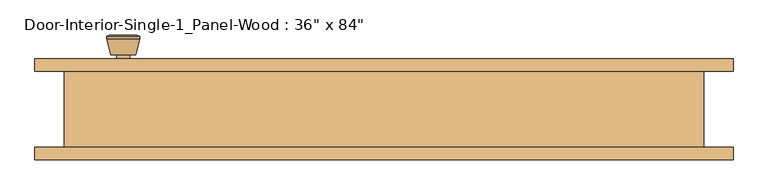
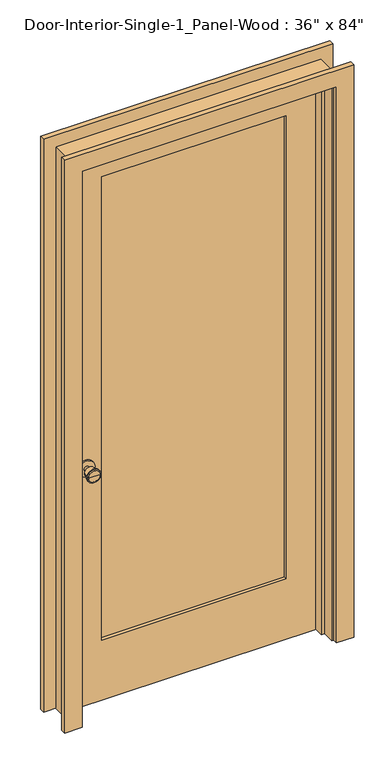
"""IFC4 building model written with IfcOpenShell, lengths in millimetres: door geometry."""

from ifc_helpers import new_model, si_unit, point, frame, frame_2d, origin, place, context, project, spatial, polyline, circle_curve, trimmed, segment, composite_curve, outline, extrude, faceted_brep, source, transform, mapped, element, save
from ifc_brep_helpers import plane_surface, cylinder_surface, revolved_surface, advanced_brep


def door_3c6ab76a(model_context):
    return source(origin(), model_context, "Body", "SolidModel", [
        advanced_brep(
        [(-393.7, 13.05, 914.4), (-383.7, 13.05, 914.4), (-403.7, 13.05, 914.4), (-373.2241324, -35.95, 914.4), (-393.7, -35.95, 914.4), (-414.1758676, -35.95, 914.4), (-368.7, -34.1221319, 914.4), (-418.7, -34.1221319, 914.4), (-368.7, -30.6584537, 914.4), (-418.7, -30.6584537, 914.4), (-375.063764, -5.95, 914.4), (-412.336236, -5.95, 914.4), (-383.7, -5.95, 914.4), (-403.7, -5.95, 914.4)],
        [
            (0, 1),
            (1, 2, circle_curve(frame((-393.7, 13.05, 914.4), z_axis=(0.0, 1.0, 0.0), x_axis=(-1.0, 0.0, 0.0)), 10.0)),
            (2, 0),
            (2, 1, circle_curve(frame((-393.7, 13.05, 914.4), z_axis=(0.0, 1.0, 0.0), x_axis=(-1.0, 0.0, 0.0)), 10.0)),
            (3, 4),
            (4, 5),
            (5, 3, circle_curve(frame((-393.7, -35.95, 914.4), z_axis=(0.0, -1.0, 0.0), x_axis=(-1.0, 0.0, 0.0)), 20.4758676)),
            (3, 5, circle_curve(frame((-393.7, -35.95, 914.4), z_axis=(0.0, -1.0, 0.0), x_axis=(-1.0, 0.0, 0.0)), 20.4758676)),
            (6, 3),
            (5, 7),
            (7, 6, circle_curve(frame((-393.7, -34.1221319, 914.4), z_axis=(0.0, -1.0, 0.0), x_axis=(-1.0, 0.0, 0.0)), 25.0)),
            (6, 7, circle_curve(frame((-393.7, -34.1221319, 914.4), z_axis=(0.0, -1.0, 0.0), x_axis=(-1.0, 0.0, 0.0)), 25.0)),
            (8, 6),
            (7, 9),
            (9, 8, circle_curve(frame((-393.7, -30.6584537, 914.4), z_axis=(0.0, -1.0, 0.0), x_axis=(-1.0, 0.0, 0.0)), 25.0)),
            (8, 9, circle_curve(frame((-393.7, -30.6584537, 914.4), z_axis=(0.0, -1.0, 0.0), x_axis=(-1.0, 0.0, 0.0)), 25.0)),
            (10, 8),
            (9, 11),
            (11, 10, circle_curve(frame((-393.7, -5.95, 914.4), z_axis=(0.0, -1.0, 0.0), x_axis=(-1.0, 0.0, 0.0)), 18.636236)),
            (10, 11, circle_curve(frame((-393.7, -5.95, 914.4), z_axis=(0.0, -1.0, 0.0), x_axis=(-1.0, 0.0, 0.0)), 18.636236)),
            (12, 10),
            (11, 13),
            (13, 12, circle_curve(frame((-393.7, -5.95, 914.4), z_axis=(0.0, -1.0, 0.0), x_axis=(-1.0, 0.0, 0.0)), 10.0)),
            (12, 13, circle_curve(frame((-393.7, -5.95, 914.4), z_axis=(0.0, -1.0, 0.0), x_axis=(-1.0, 0.0, 0.0)), 10.0)),
            (1, 12),
            (13, 2),
        ],
        [
            plane_surface(frame((-393.7, 13.05, 914.4), z_axis=(0.0, 1.0, 0.0), x_axis=(-1.0, 0.0, 0.0))),
            plane_surface(frame((-393.7, -35.95, 914.4), z_axis=(0.0, -1.0, 0.0), x_axis=(-1.0, 0.0, 0.0))),
            revolved_surface(polyline([(-414.1758676, -35.95, 914.4), (-418.7, -34.1221319, 914.4)]), (-393.7, 13.05, 914.4), (0.0, 1.0, 0.0)),
            cylinder_surface(frame((-393.7, 13.05, 914.4), z_axis=(0.0, 1.0, 0.0), x_axis=(-1.0, 0.0, 0.0)), 25.0),
            revolved_surface(polyline([(-418.7, -30.6584537, 914.4), (-412.336236, -5.95, 914.4)]), (-393.7, 13.05, 914.4), (0.0, 1.0, 0.0)),
            plane_surface(frame((-393.7, -5.95, 914.4), z_axis=(0.0, 1.0, 0.0), x_axis=(-1.0, 0.0, 0.0))),
            cylinder_surface(frame((-393.7, 13.05, 914.4), z_axis=(0.0, 1.0, 0.0), x_axis=(-1.0, 0.0, 0.0)), 10.0),
        ],
        [
            (0, [[1, 2, 3]]),
            (0, [[-3, 4, -1]]),
            (1, [[5, 6, 7]]),
            (1, [[-6, -5, 8]]),
            (2, [[9, -7, 10, 11]]),
            (2, [[-10, -8, -9, 12]]),
            (3, [[13, -11, 14, 15]]),
            (3, [[-14, -12, -13, 16]]),
            (4, [[17, -15, 18, 19]]),
            (4, [[-18, -16, -17, 20]]),
            (5, [[21, -19, 22, 23]]),
            (5, [[-22, -20, -21, 24]]),
            (6, [[25, -23, 26, -2]]),
            (6, [[-26, -24, -25, -4]]),
        ],
    ),
        extrude(outline(composite_curve([segment(trimmed(circle_curve(frame_2d((914.4, -393.7)), 30.0), [point((914.4, -423.7))], [point((914.4, -363.7))], False, "CARTESIAN"), True, "CONTINUOUS"), segment(trimmed(circle_curve(frame_2d((914.4, -393.7)), 30.0), [point((914.4, -363.7))], [point((914.4, -423.7))], False, "CARTESIAN"), True, "CONTINUOUS")], self_intersect=False)), frame((0.0, 13.05, 0.0), z_axis=(0.0, 1.0, 0.0), x_axis=(0.0, 0.0, 1.0)), (0.0, 0.0, 1.0), 6.0),
        advanced_brep(
        [(-393.7, 59.975, 914.4), (-403.7, 59.975, 914.4), (-383.7, 59.975, 914.4), (-373.2241324, 108.975, 914.4), (-414.1758676, 108.975, 914.4), (-393.7, 108.975, 914.4), (-368.7, 107.1471319, 914.4), (-418.7, 107.1471319, 914.4), (-368.7, 103.6834537, 914.4), (-418.7, 103.6834537, 914.4), (-375.063764, 78.975, 914.4), (-412.336236, 78.975, 914.4), (-383.7, 78.975, 914.4), (-403.7, 78.975, 914.4)],
        [
            (0, 1),
            (1, 2, circle_curve(frame((-393.7, 59.975, 914.4), z_axis=(0.0, -1.0, 0.0), x_axis=(-1.0, 0.0, 0.0)), 10.0)),
            (2, 0),
            (2, 1, circle_curve(frame((-393.7, 59.975, 914.4), z_axis=(0.0, -1.0, 0.0), x_axis=(-1.0, 0.0, 0.0)), 10.0)),
            (3, 4, circle_curve(frame((-393.7, 108.975, 914.4), z_axis=(0.0, 1.0, 0.0), x_axis=(-1.0, 0.0, 0.0)), 20.4758676)),
            (4, 5),
            (5, 3),
            (4, 3, circle_curve(frame((-393.7, 108.975, 914.4), z_axis=(0.0, 1.0, 0.0), x_axis=(-1.0, 0.0, 0.0)), 20.4758676)),
            (6, 7, circle_curve(frame((-393.7, 107.1471319, 914.4), z_axis=(0.0, 1.0, 0.0), x_axis=(-1.0, 0.0, 0.0)), 25.0)),
            (7, 4),
            (3, 6),
            (7, 6, circle_curve(frame((-393.7, 107.1471319, 914.4), z_axis=(0.0, 1.0, 0.0), x_axis=(-1.0, 0.0, 0.0)), 25.0)),
            (8, 9, circle_curve(frame((-393.7, 103.6834537, 914.4), z_axis=(0.0, 1.0, 0.0), x_axis=(-1.0, 0.0, 0.0)), 25.0)),
            (9, 7),
            (6, 8),
            (9, 8, circle_curve(frame((-393.7, 103.6834537, 914.4), z_axis=(0.0, 1.0, 0.0), x_axis=(-1.0, 0.0, 0.0)), 25.0)),
            (10, 11, circle_curve(frame((-393.7, 78.975, 914.4), z_axis=(0.0, 1.0, 0.0), x_axis=(-1.0, 0.0, 0.0)), 18.636236)),
            (11, 9),
            (8, 10),
            (11, 10, circle_curve(frame((-393.7, 78.975, 914.4), z_axis=(0.0, 1.0, 0.0), x_axis=(-1.0, 0.0, 0.0)), 18.636236)),
            (12, 13, circle_curve(frame((-393.7, 78.975, 914.4), z_axis=(0.0, 1.0, 0.0), x_axis=(-1.0, 0.0, 0.0)), 10.0)),
            (13, 11),
            (10, 12),
            (13, 12, circle_curve(frame((-393.7, 78.975, 914.4), z_axis=(0.0, 1.0, 0.0), x_axis=(-1.0, 0.0, 0.0)), 10.0)),
            (1, 13),
            (12, 2),
        ],
        [
            plane_surface(frame((-393.7, 59.975, 914.4), z_axis=(0.0, -1.0, 0.0), x_axis=(-1.0, 0.0, 0.0))),
            plane_surface(frame((-393.7, 108.975, 914.4), z_axis=(0.0, 1.0, 0.0), x_axis=(-1.0, 0.0, 0.0))),
            revolved_surface(polyline([(-414.1758676, 108.975, 914.4), (-418.7, 107.1471319, 914.4)]), (-393.7, 59.975, 914.4), (0.0, -1.0, 0.0)),
            cylinder_surface(frame((-393.7, 59.975, 914.4), z_axis=(0.0, -1.0, 0.0), x_axis=(-1.0, 0.0, 0.0)), 25.0),
            revolved_surface(polyline([(-418.7, 103.6834537, 914.4), (-412.336236, 78.975, 914.4)]), (-393.7, 59.975, 914.4), (0.0, -1.0, 0.0)),
            plane_surface(frame((-393.7, 78.975, 914.4), z_axis=(0.0, -1.0, 0.0), x_axis=(-1.0, 0.0, 0.0))),
            cylinder_surface(frame((-393.7, 59.975, 914.4), z_axis=(0.0, -1.0, 0.0), x_axis=(-1.0, 0.0, 0.0)), 10.0),
        ],
        [
            (0, [[1, 2, 3]]),
            (0, [[-3, 4, -1]]),
            (1, [[5, 6, 7]]),
            (1, [[8, -7, -6]]),
            (2, [[9, 10, -5, 11]]),
            (2, [[12, -11, -8, -10]]),
            (3, [[13, 14, -9, 15]]),
            (3, [[16, -15, -12, -14]]),
            (4, [[17, 18, -13, 19]]),
            (4, [[20, -19, -16, -18]]),
            (5, [[21, 22, -17, 23]]),
            (5, [[24, -23, -20, -22]]),
            (6, [[-2, 25, -21, 26]]),
            (6, [[-4, -26, -24, -25]]),
        ],
    ),
        extrude(outline(composite_curve([segment(trimmed(circle_curve(frame_2d((914.4, -393.7)), 30.0), [point((914.4, -423.7))], [point((914.4, -363.7))], False, "CARTESIAN"), True, "CONTINUOUS"), segment(trimmed(circle_curve(frame_2d((914.4, -393.7)), 30.0), [point((914.4, -363.7))], [point((914.4, -423.7))], False, "CARTESIAN"), True, "CONTINUOUS")], self_intersect=False)), frame((0.0, 53.975, 0.0), z_axis=(0.0, 1.0, 0.0), x_axis=(0.0, 0.0, 1.0)), (0.0, 0.0, 1.0), 6.0),
        faceted_brep([(482.6, 53.975, 0.0), (482.6, -60.325, 0.0), (457.2, -60.325, 0.0), (457.2, -15.875, 0.0), (444.5, -15.875, 0.0), (444.5, 19.05, 0.0), (457.2, 19.05, 0.0), (457.2, 53.975, 0.0), (482.6, 53.975, 2159.0), (482.6, -60.325, 2159.0), (-482.6, -60.325, 2159.0), (-482.6, -60.325, 0.0), (-457.2, -60.325, 0.0), (-457.2, -60.325, 2133.6), (457.2, -60.325, 2133.6), (457.2, -15.875, 2133.6), (-457.2, -15.875, 2133.6), (-457.2, -15.875, 0.0), (-444.5, -15.875, 0.0), (-444.5, -15.875, 2120.9), (444.5, -15.875, 2120.9), (444.5, 19.05, 2120.9), (-444.5, 19.05, 2120.9), (-444.5, 19.05, 0.0), (-457.2, 19.05, 0.0), (-457.2, 19.05, 2133.6), (457.2, 19.05, 2133.6), (457.2, 53.975, 2133.6), (-457.2, 53.975, 2133.6), (-457.2, 53.975, 0.0), (-482.6, 53.975, 0.0), (-482.6, 53.975, 2159.0)], [[[0, 1, 2, 3, 4, 5, 6, 7]], [[1, 0, 8, 9]], [[2, 1, 9, 10, 11, 12, 13, 14]], [[3, 2, 14, 15]], [[4, 3, 15, 16, 17, 18, 19, 20]], [[5, 4, 20, 21]], [[6, 5, 21, 22, 23, 24, 25, 26]], [[7, 6, 26, 27]], [[0, 7, 27, 28, 29, 30, 31, 8]], [[9, 8, 31, 10]], [[15, 14, 13, 16]], [[21, 20, 19, 22]], [[27, 26, 25, 28]], [[30, 29, 24, 23, 18, 17, 12, 11]], [[10, 31, 30, 11]], [[16, 13, 12, 17]], [[22, 19, 18, 23]], [[28, 25, 24, 29]]]),
        extrude(outline(polyline([(2133.6, -457.2), (0.0, -457.2), (0.0, 457.2), (2133.6, 457.2), (2133.6, -457.2)]), holes=[polyline([(2014.5375, -336.55), (2014.5375, 336.55), (231.775, 336.55), (231.775, -336.55), (2014.5375, -336.55)])]), frame((0.0, 19.05, 0.0), z_axis=(0.0, 1.0, 0.0), x_axis=(0.0, 0.0, 1.0)), (0.0, 0.0, 1.0), 34.925),
        extrude(outline(polyline([(336.55, 30.6916667), (-336.55, 30.6916667), (-336.55, 42.3333333), (336.55, 42.3333333), (336.55, 30.6916667)])), frame((0.0, 0.0, 231.775), z_axis=(0.0, 0.0, 1.0), x_axis=(1.0, 0.0, 0.0)), (0.0, 0.0, 1.0), 1782.7625),
        extrude(outline(polyline([(0.0, 463.55), (0.0, 527.05), (2203.45, 527.05), (2203.45, -527.05), (0.0, -527.05), (0.0, -463.55), (2139.95, -463.55), (2139.95, 463.55), (0.0, 463.55)])), frame((0.0, 53.975, 0.0), z_axis=(0.0, 1.0, 0.0), x_axis=(0.0, 0.0, 1.0)), (0.0, 0.0, 1.0), 19.05),
        extrude(outline(polyline([(0.0, 463.55), (0.0, 527.05), (2203.45, 527.05), (2203.45, -527.05), (0.0, -527.05), (0.0, -463.55), (2139.95, -463.55), (2139.95, 463.55), (0.0, 463.55)])), frame((0.0, -79.375, 0.0), z_axis=(0.0, 1.0, 0.0), x_axis=(0.0, 0.0, 1.0)), (0.0, 0.0, 1.0), 19.05),
    ])


if __name__ == "__main__":
    model = new_model("IFC4")
    model_context = context("Model", 3, world=origin())
    ifc_project = project(units=[si_unit("LENGTHUNIT", "METRE", prefix="MILLI")], contexts=[model_context])
    site = spatial("IfcSite", under=ifc_project)
    building = spatial("IfcBuilding", under=site)
    placement = place(None, origin())
    door_shape = door_3c6ab76a(model_context)
    element("IfcDoor", 1, ObjectType="Door-Interior-Single-1_Panel-Wood : 36\" x 84\"", at=placement, inside=building, context=model_context, shape_type="MappedRepresentation", body=[
        mapped(door_shape, transform((0.0, 0.0, 0.0), x_axis=(1.0, 0.0, 0.0), y_axis=(0.0, 1.0, 0.0), z_axis=(0.0, 0.0, 1.0))),
    ])
    save(model, "model.ifc")

# Revit data of these elements
# Type "Door-Interior-Single-1_Panel-Wood : 36\" x 84\""
#   Type Mark = "15"
#   Assembly Code = "C1020300"
#   Analytic Construction = "Wooden"
#   Top Rail = 0' - 4 11/16"
#   Thickness = 0' - 1 3/8"
#   Thermal Resistance (R) = 2.5876 (h·ft²·°F)/BTU
#   Swing Angle [instance default] = 90.00°
#   Stiles = 0' - 4 3/4"
#   Rough Width = 3' - 2"
#   Rough Height = 7' - 1"
#   Height = 7' - 0"
#   Width = 3' - 0"
#   Heat Transfer Coefficient (U) = 0.3865 BTU/(h·ft²·°F)
#   Bottom Rail = 0' - 9 1/8"
#   Trim Material = Cherry
#   Panel Material = Cherry
#   Frame Material = Cherry
#   Door Handle Material = Aluminum
#   Visual Light Transmittance = 0
#   Solar Heat Gain Coefficient = 0
#   Wall Closure = (empty or 0)
#   Function = (empty or 0)
# Element 1 (IfcDoor, "Door-Interior-Single-1_Panel-Wood : 36\" x 84\"")
#   Materials on its faces: "Cherry", "Aluminum"
# Materials
#   "Cherry": class "Wood", colour RGB 226 177 128, transparency 0, Description = "Prunus Serotina", Cost = 0
#   "Aluminum": class "Metal", colour RGB 247 247 247, transparency 0, Description = "Aluminum 6061", Cost = 0
